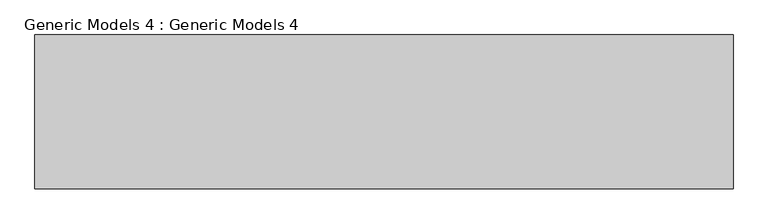
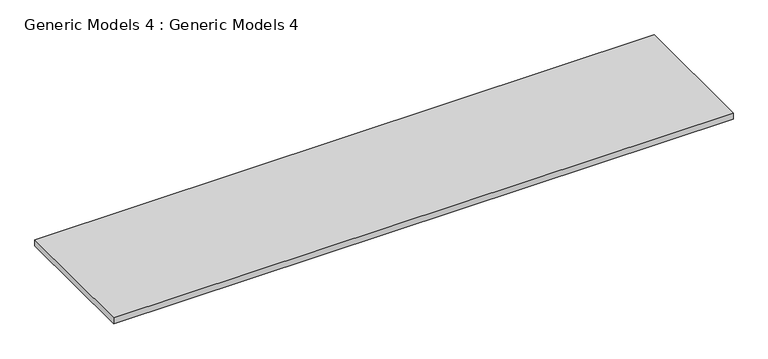
"""IFC4 building model written with IfcOpenShell, lengths in millimetres: proxy geometry, Generic Models 4 : Generic Models 4."""

from ifc_helpers import new_model, si_unit, frame, origin, place, context, project, spatial, polyline, outline, extrude, source, transform, mapped, element, save


def generic_models_4_generic_models_4_ada6ec20(model_context):
    return source(origin(), model_context, "Body", "SweptSolid", [
        extrude(outline(polyline([(-8961.0740184, -10090.8448149), (5669.3259816, -10090.8448149), (5669.3259816, -13316.1257992), (-8961.0740184, -13316.1257992), (-8961.0740184, -10090.8448149)])), frame((0.0, 0.0, -152.4), z_axis=(0.0, 0.0, 1.0), x_axis=(1.0, 0.0, 0.0)), (0.0, 0.0, 1.0), 152.4),
    ])


if __name__ == "__main__":
    model = new_model("IFC4")
    model_context = context("Model", 3, world=origin())
    ifc_project = project(units=[si_unit("LENGTHUNIT", "METRE", prefix="MILLI")], contexts=[model_context])
    site = spatial("IfcSite", under=ifc_project)
    building = spatial("IfcBuilding", under=site)
    placement = place(None, origin())
    generic_models_4_generic_models_4_shape = generic_models_4_generic_models_4_ada6ec20(model_context)
    element("IfcBuildingElementProxy", 1, Name="Generic Models 4 : Generic Models 4", ObjectType="Generic Models 4 : Generic Models 4", at=placement, inside=building, context=model_context, shape_type="MappedRepresentation", body=[
        mapped(generic_models_4_generic_models_4_shape, transform((0.0, 0.0, 0.0), x_axis=(1.0, 0.0, 0.0), y_axis=(0.0, 1.0, 0.0), z_axis=(0.0, 0.0, 1.0))),
    ])
    save(model, "model.ifc")
